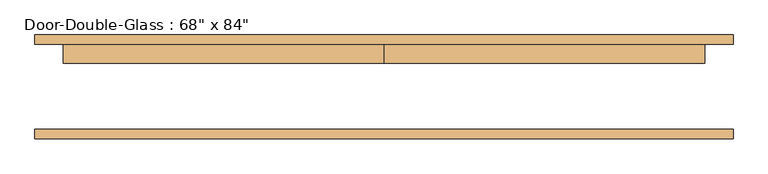
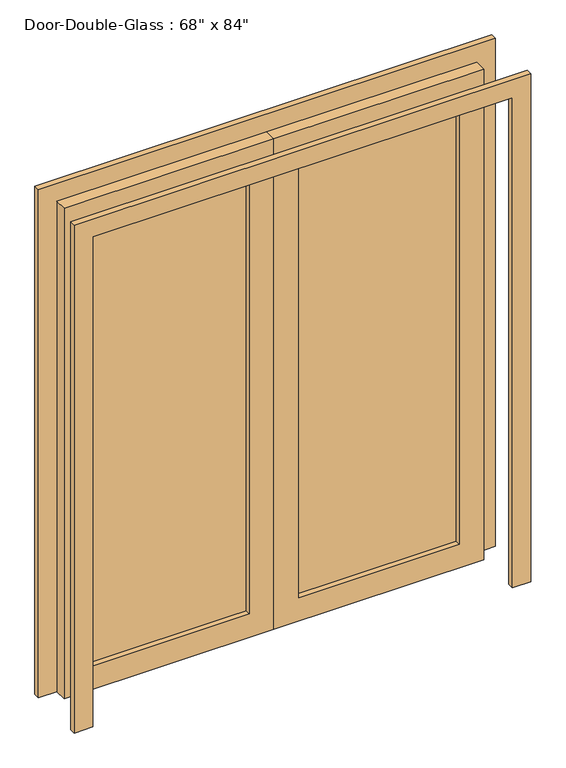
"""IFC4 building model written with IfcOpenShell, lengths in millimetres: door geometry."""

from ifc_helpers import new_model, si_unit, frame, origin, place, context, project, spatial, polyline, outline, extrude, source, transform, mapped, element, save


def door_e52a3823(model_context):
    return source(origin(), model_context, "Body", "SweptSolid", [
        extrude(outline(polyline([(2133.6, 863.6), (2133.6, 0.0), (0.0, 0.0), (0.0, 863.6), (2133.6, 863.6)]), holes=[polyline([(2032.0, 762.0), (101.6, 762.0), (101.6, 101.6), (2032.0, 101.6), (2032.0, 762.0)])]), frame((0.0, 65.88125, 0.0), z_axis=(0.0, 1.0, 0.0), x_axis=(0.0, 0.0, 1.0)), (0.0, 0.0, 1.0), 50.8),
        extrude(outline(polyline([(2133.6, -863.6), (0.0, -863.6), (0.0, 0.0), (2133.6, 0.0), (2133.6, -863.6)]), holes=[polyline([(2032.0, -762.0), (2032.0, -101.6), (101.6, -101.6), (101.6, -762.0), (2032.0, -762.0)])]), frame((0.0, 65.88125, 0.0), z_axis=(0.0, 1.0, 0.0), x_axis=(0.0, 0.0, 1.0)), (0.0, 0.0, 1.0), 50.8),
        extrude(outline(polyline([(-762.0, 94.45625), (-101.6, 94.45625), (-101.6, 88.10625), (-762.0, 88.10625), (-762.0, 94.45625)])), frame((0.0, 0.0, 101.6), z_axis=(0.0, 0.0, 1.0), x_axis=(1.0, 0.0, 0.0)), (0.0, 0.0, 1.0), 1930.4),
        extrude(outline(polyline([(101.6, 94.45625), (762.0, 94.45625), (762.0, 88.10625), (101.6, 88.10625), (101.6, 94.45625)])), frame((0.0, 0.0, 101.6), z_axis=(0.0, 0.0, 1.0), x_axis=(1.0, 0.0, 0.0)), (0.0, 0.0, 1.0), 1930.4),
        extrude(outline(polyline([(0.0, 939.8), (2209.8, 939.8), (2209.8, -939.8), (0.0, -939.8), (0.0, -863.6), (2133.6, -863.6), (2133.6, 863.6), (0.0, 863.6), (0.0, 939.8)])), frame((0.0, -137.31875, 0.0), z_axis=(0.0, 1.0, 0.0), x_axis=(0.0, 0.0, 1.0)), (0.0, 0.0, 1.0), 25.4),
        extrude(outline(polyline([(0.0, 939.8), (2209.8, 939.8), (2209.8, -939.8), (0.0, -939.8), (0.0, -863.6), (2133.6, -863.6), (2133.6, 863.6), (0.0, 863.6), (0.0, 939.8)])), frame((0.0, 116.68125, 0.0), z_axis=(0.0, 1.0, 0.0), x_axis=(0.0, 0.0, 1.0)), (0.0, 0.0, 1.0), 25.4),
    ])


if __name__ == "__main__":
    model = new_model("IFC4")
    model_context = context("Model", 3, world=origin())
    ifc_project = project(units=[si_unit("LENGTHUNIT", "METRE", prefix="MILLI")], contexts=[model_context])
    site = spatial("IfcSite", under=ifc_project)
    building = spatial("IfcBuilding", under=site)
    placement = place(None, origin())
    door_shape = door_e52a3823(model_context)
    element("IfcDoor", 1, ObjectType="Door-Double-Glass : 68\" x 84\"", at=placement, inside=building, context=model_context, shape_type="MappedRepresentation", body=[
        mapped(door_shape, transform((0.0, 0.0, 0.0), x_axis=(1.0, 0.0, 0.0), y_axis=(0.0, 1.0, 0.0), z_axis=(0.0, 0.0, 1.0))),
    ])
    save(model, "model.ifc")

# Revit data of these elements
# Type "Door-Double-Glass : 68\" x 84\""
#   Type Mark = "11"
#   Construction Type Id = "opn-d45"
#   Assembly Code = "C1020"
#   Analytic Construction = "Wood frame, double glass door "
#   W = 2' - 10"
#   Thickness = 0' - 2"
#   Thermal Resistance (R) = 1.8150 (h·ft²·°F)/BTU
#   Swing Angle [instance default] = 90.00°
#   Heat Transfer Coefficient (U) = 0.5510 BTU/(h·ft²·°F)
#   Height = 7' - 0"
#   Bottom Rail = 0' - 4"
#   Top Rail = 0' - 4"
#   Stiles = 0' - 4"
#   Trim Projection = 0' - 1"
#   Trim Width = 0' - 3"
#   Width = 5' - 8"
#   Define Thermal Properties by = 1
#   Glazing = Glass
#   Panel Material = Wood - Birch - Solid Stained Light Low Gloss
#   Trim Material = Paint - Sienna
#   Visual Light Transmittance = 0
#   Solar Heat Gain Coefficient = 0
#   Function = (empty or 0)
#   Wall Closure = (empty or 0)
# Element 1 (IfcDoor, "Door-Double-Glass : 68\" x 84\"")
#   Materials on its faces: "Wood - Birch - Solid Stained Light Low Gloss", "Paint - Sienna", "Glass"
# Materials
#   "Glass": class "Glass", colour RGB 0 128 192, transparency 0.75, Description = "Soda Lime Glass", Cost = 0
#   "Wood - Birch - Solid Stained Light Low Gloss": class "Wood", colour RGB 210 159 95, transparency 0, Cost = 0
#   "Paint - Sienna": colour RGB 118 70 51, transparency 0, Cost = 0
